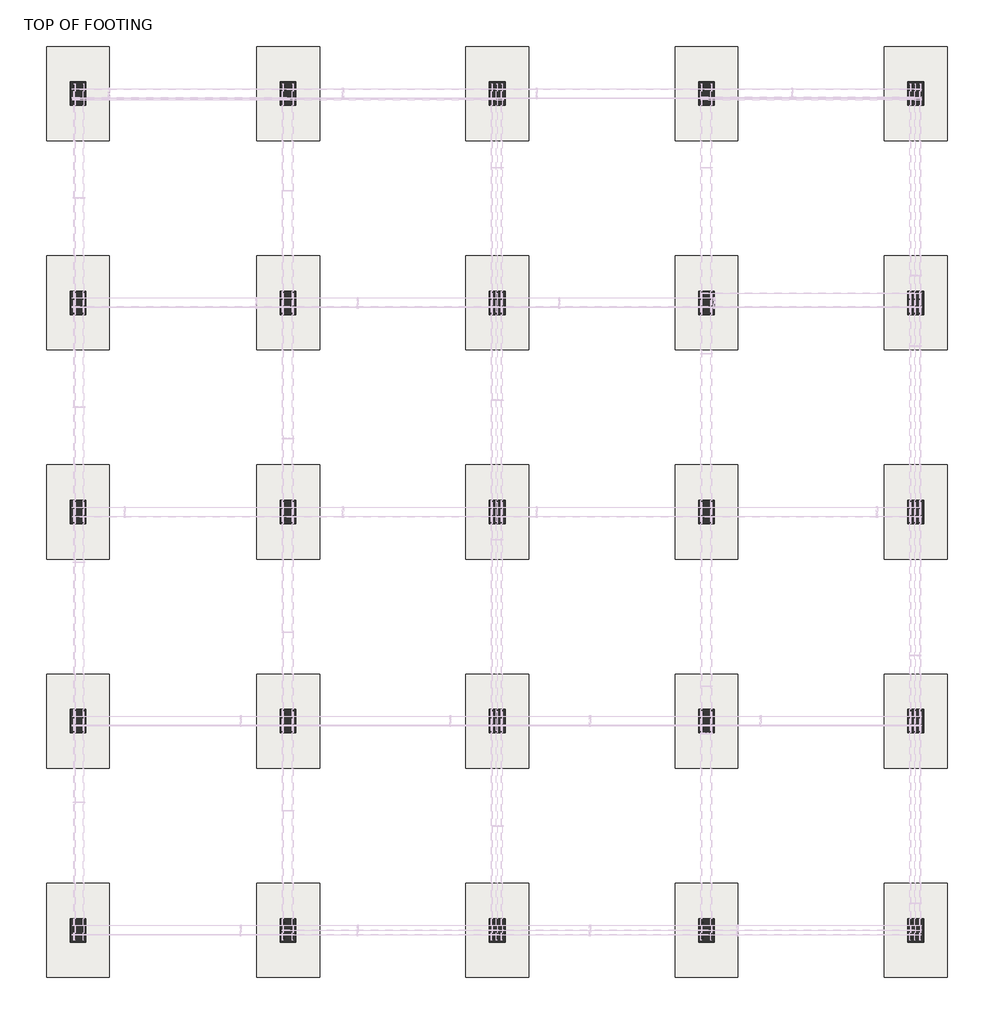
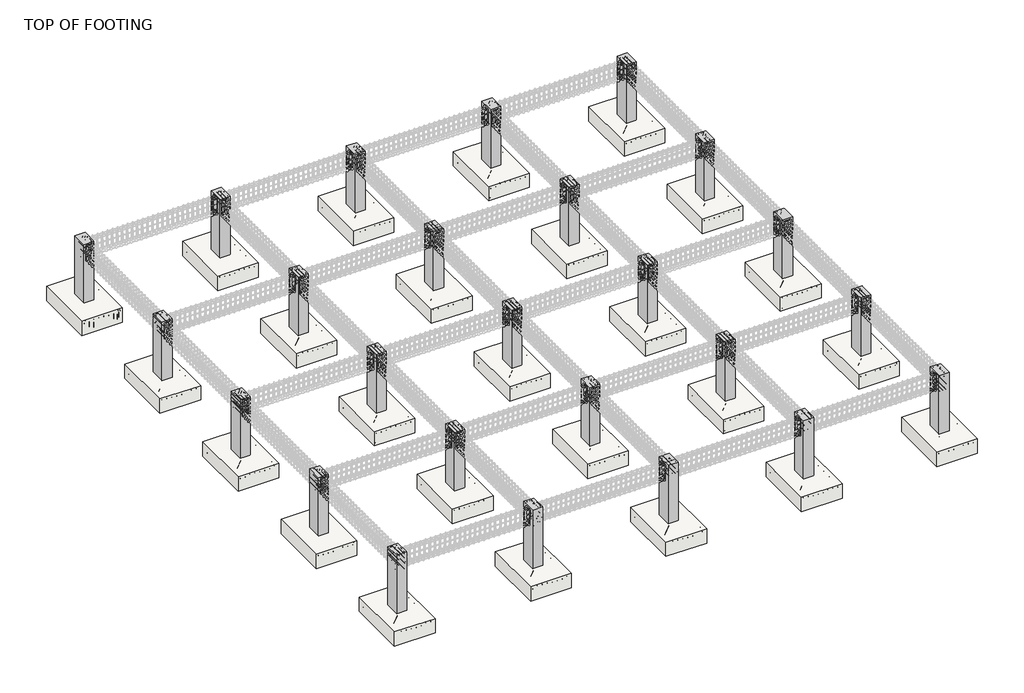
# One storey, part 1 of 21: 25 columns, 25 slabs.
"""IFC4 building model written with IfcOpenShell, lengths in millimetres."""

from ifc_helpers import new_model, si_unit, frame, origin, place, context, project, spatial, polyline, outline, extrude, faceted_brep, transform, mapped, element, save
from components import m_footing_rectangular_1800_x_1200_x_450mm_16ba7ea5

model = new_model("IFC4")

# Units and contexts
model_context = context("Model", 3, world=origin())
ifc_project = project(units=[si_unit("LENGTHUNIT", "METRE", prefix="MILLI")], contexts=[model_context])

# Site, building, storey
site = spatial("IfcSite", under=ifc_project)
building = spatial("IfcBuilding", under=site)
storey = spatial("IfcBuildingStorey", under=building, Name="TOP OF FOOTING", Elevation=-1828.8)

# Columns
placement = place(None, origin())
element("IfcColumn", 1, ObjectType="M_Concrete-Rectangular-Column : 300 x 450mm", at=placement, inside=storey, context=model_context, shape_type="SweptSolid", body=[
    extrude(outline(polyline([(-13671.9084825, 15814.5386958), (-13671.9084825, 15364.5386958), (-13971.9084825, 15364.5386958), (-13971.9084825, 15814.5386958), (-13671.9084825, 15814.5386958)])), frame((0.0, 0.0, -1828.8), z_axis=(0.0, 0.0, 1.0), x_axis=(1.0, 0.0, 0.0)), (0.0, 0.0, 1.0), 1828.8),
])
element("IfcColumn", 2, ObjectType="M_Concrete-Rectangular-Column : 300 x 450mm", at=placement, inside=storey, context=model_context, shape_type="Brep", body=[
    faceted_brep([(-9652.1813539, 15814.5386958, -1828.8), (-9652.1813539, 15364.5386958, -1828.8), (-9952.1813539, 15364.5386958, -1828.8), (-9952.1813539, 15814.5386958, -1828.8), (-9652.1813539, 15814.5386958, 0.0), (-9652.1813539, 15439.5386958, 0.0), (-9652.1813539, 15364.5386958, 0.0), (-9952.1813539, 15364.5386958, 0.0), (-9952.1813539, 15439.5386958, 0.0), (-9952.1813539, 15814.5386958, 0.0)], [[[0, 1, 2, 3]], [[4, 5, 6, 1, 0]], [[6, 7, 2, 1]], [[7, 8, 9, 3, 2]], [[9, 4, 0, 3]], [[4, 9, 8, 7, 6, 5]]]),
])
element("IfcColumn", 3, ObjectType="M_Concrete-Rectangular-Column : 300 x 450mm", at=placement, inside=storey, context=model_context, shape_type="Brep", body=[
    faceted_brep([(-5652.1813539, 15814.5386958, -1828.8), (-5652.1813539, 15364.5386958, -1828.8), (-5952.1813539, 15364.5386958, -1828.8), (-5952.1813539, 15814.5386958, -1828.8), (-5652.1813539, 15814.5386958, 0.0), (-5652.1813539, 15439.5386958, 0.0), (-5652.1813539, 15364.5386958, 0.0), (-5952.1813539, 15364.5386958, 0.0), (-5952.1813539, 15439.5386958, 0.0), (-5952.1813539, 15814.5386958, 0.0)], [[[0, 1, 2, 3]], [[4, 5, 6, 1, 0]], [[6, 7, 2, 1]], [[7, 8, 9, 3, 2]], [[9, 4, 0, 3]], [[4, 9, 8, 7, 6, 5]]]),
])
element("IfcColumn", 4, ObjectType="M_Concrete-Rectangular-Column : 300 x 450mm", at=placement, inside=storey, context=model_context, shape_type="Brep", body=[
    faceted_brep([(-1652.1813539, 15814.5386958, -1828.8), (-1652.1813539, 15364.5386958, -1828.8), (-1952.1813539, 15364.5386958, -1828.8), (-1952.1813539, 15814.5386958, -1828.8), (-1652.1813539, 15814.5386958, 0.0), (-1652.1813539, 15439.5386958, 0.0), (-1652.1813539, 15364.5386958, 0.0), (-1952.1813539, 15364.5386958, 0.0), (-1952.1813539, 15439.5386958, 0.0), (-1952.1813539, 15814.5386958, 0.0)], [[[0, 1, 2, 3]], [[4, 5, 6, 1, 0]], [[6, 7, 2, 1]], [[7, 8, 9, 3, 2]], [[9, 4, 0, 3]], [[4, 9, 8, 7, 6, 5]]]),
])
element("IfcColumn", 5, ObjectType="M_Concrete-Rectangular-Column : 300 x 450mm", at=placement, inside=storey, context=model_context, shape_type="Brep", body=[
    faceted_brep([(2347.8186461, 15814.5386958, -1828.8), (2347.8186461, 15364.5386958, -1828.8), (2047.8186461, 15364.5386958, -1828.8), (2047.8186461, 15814.5386958, -1828.8), (2347.8186461, 15814.5386958, 0.0), (2347.8186461, 15364.5386958, 0.0), (2047.8186461, 15364.5386958, 0.0), (2047.8186461, 15439.5386958, 0.0), (2047.8186461, 15814.5386958, 0.0)], [[[0, 1, 2, 3]], [[4, 5, 1, 0]], [[5, 6, 2, 1]], [[6, 7, 8, 3, 2]], [[8, 4, 0, 3]], [[4, 8, 7, 6, 5]]]),
])
element("IfcColumn", 6, ObjectType="M_Concrete-Rectangular-Column : 300 x 450mm", at=placement, inside=storey, context=model_context, shape_type="SweptSolid", body=[
    extrude(outline(polyline([(-13671.9084825, 11814.5386958), (-13671.9084825, 11364.5386958), (-13971.9084825, 11364.5386958), (-13971.9084825, 11814.5386958), (-13671.9084825, 11814.5386958)])), frame((0.0, 0.0, -1828.8), z_axis=(0.0, 0.0, 1.0), x_axis=(1.0, 0.0, 0.0)), (0.0, 0.0, 1.0), 1828.8),
])
element("IfcColumn", 7, ObjectType="M_Concrete-Rectangular-Column : 300 x 450mm", at=placement, inside=storey, context=model_context, shape_type="Brep", body=[
    faceted_brep([(-9652.1813539, 11814.5386958, -1828.8), (-9652.1813539, 11364.5386958, -1828.8), (-9952.1813539, 11364.5386958, -1828.8), (-9952.1813539, 11814.5386958, -1828.8), (-9652.1813539, 11814.5386958, 0.0), (-9652.1813539, 11739.5386958, 0.0), (-9652.1813539, 11439.5386958, 0.0), (-9652.1813539, 11364.5386958, 0.0), (-9952.1813539, 11364.5386958, 0.0), (-9952.1813539, 11439.5386958, 0.0), (-9952.1813539, 11739.5386958, 0.0), (-9952.1813539, 11814.5386958, 0.0)], [[[0, 1, 2, 3]], [[4, 5, 6, 7, 1, 0]], [[7, 8, 2, 1]], [[8, 9, 10, 11, 3, 2]], [[11, 4, 0, 3]], [[4, 11, 10, 9, 8, 7, 6, 5]]]),
])
element("IfcColumn", 8, ObjectType="M_Concrete-Rectangular-Column : 300 x 450mm", at=placement, inside=storey, context=model_context, shape_type="Brep", body=[
    faceted_brep([(-5652.1813539, 11814.5386958, -1828.8), (-5652.1813539, 11364.5386958, -1828.8), (-5952.1813539, 11364.5386958, -1828.8), (-5952.1813539, 11814.5386958, -1828.8), (-5652.1813539, 11814.5386958, 0.0), (-5652.1813539, 11739.5386958, 0.0), (-5652.1813539, 11439.5386958, 0.0), (-5652.1813539, 11364.5386958, 0.0), (-5952.1813539, 11364.5386958, 0.0), (-5952.1813539, 11439.5386958, 0.0), (-5952.1813539, 11739.5386958, 0.0), (-5952.1813539, 11814.5386958, 0.0)], [[[0, 1, 2, 3]], [[4, 5, 6, 7, 1, 0]], [[7, 8, 2, 1]], [[8, 9, 10, 11, 3, 2]], [[11, 4, 0, 3]], [[4, 11, 10, 9, 8, 7, 6, 5]]]),
])
element("IfcColumn", 9, ObjectType="M_Concrete-Rectangular-Column : 300 x 450mm", at=placement, inside=storey, context=model_context, shape_type="Brep", body=[
    faceted_brep([(-1652.1813539, 11814.5386958, -1828.8), (-1652.1813539, 11364.5386958, -1828.8), (-1952.1813539, 11364.5386958, -1828.8), (-1952.1813539, 11814.5386958, -1828.8), (-1652.1813539, 11814.5386958, 0.0), (-1652.1813539, 11739.5386958, 0.0), (-1652.1813539, 11419.5386958, 0.0), (-1652.1813539, 11364.5386958, 0.0), (-1952.1813539, 11364.5386958, 0.0), (-1952.1813539, 11439.5386958, 0.0), (-1952.1813539, 11739.5386958, 0.0), (-1952.1813539, 11814.5386958, 0.0)], [[[0, 1, 2, 3]], [[4, 5, 6, 7, 1, 0]], [[7, 8, 2, 1]], [[8, 9, 10, 11, 3, 2]], [[11, 4, 0, 3]], [[4, 11, 10, 9, 8, 7, 6, 5]]]),
])
element("IfcColumn", 10, ObjectType="M_Concrete-Rectangular-Column : 300 x 450mm", at=placement, inside=storey, context=model_context, shape_type="Brep", body=[
    faceted_brep([(2347.8186461, 11814.5386958, -1828.8), (2347.8186461, 11364.5386958, -1828.8), (2047.8186461, 11364.5386958, -1828.8), (2047.8186461, 11814.5386958, -1828.8), (2347.8186461, 11814.5386958, 0.0), (2347.8186461, 11774.5386958, 0.0), (2347.8186461, 11364.5386958, 0.0), (2047.8186461, 11364.5386958, 0.0), (2047.8186461, 11419.5386958, 0.0), (2047.8186461, 11739.5386958, 0.0), (2047.8186461, 11814.5386958, 0.0)], [[[0, 1, 2, 3]], [[4, 5, 6, 1, 0]], [[6, 7, 2, 1]], [[7, 8, 9, 10, 3, 2]], [[10, 4, 0, 3]], [[4, 10, 9, 8, 7, 6, 5]]]),
])
element("IfcColumn", 11, ObjectType="M_Concrete-Rectangular-Column : 300 x 450mm", at=placement, inside=storey, context=model_context, shape_type="SweptSolid", body=[
    extrude(outline(polyline([(-13671.9084825, 7814.5386958), (-13671.9084825, 7364.5386958), (-13971.9084825, 7364.5386958), (-13971.9084825, 7814.5386958), (-13671.9084825, 7814.5386958)])), frame((0.0, 0.0, -1828.8), z_axis=(0.0, 0.0, 1.0), x_axis=(1.0, 0.0, 0.0)), (0.0, 0.0, 1.0), 1828.8),
])
element("IfcColumn", 12, ObjectType="M_Concrete-Rectangular-Column : 300 x 450mm", at=placement, inside=storey, context=model_context, shape_type="Brep", body=[
    faceted_brep([(-9652.1813539, 7814.5386958, -1828.8), (-9652.1813539, 7364.5386958, -1828.8), (-9952.1813539, 7364.5386958, -1828.8), (-9952.1813539, 7814.5386958, -1828.8), (-9652.1813539, 7814.5386958, 0.0), (-9652.1813539, 7739.5386958, 0.0), (-9652.1813539, 7439.5386958, 0.0), (-9652.1813539, 7364.5386958, 0.0), (-9952.1813539, 7364.5386958, 0.0), (-9952.1813539, 7439.5386958, 0.0), (-9952.1813539, 7739.5386958, 0.0), (-9952.1813539, 7814.5386958, 0.0)], [[[0, 1, 2, 3]], [[4, 5, 6, 7, 1, 0]], [[7, 8, 2, 1]], [[8, 9, 10, 11, 3, 2]], [[11, 4, 0, 3]], [[4, 11, 10, 9, 8, 7, 6, 5]]]),
])
element("IfcColumn", 13, ObjectType="M_Concrete-Rectangular-Column : 300 x 450mm", at=placement, inside=storey, context=model_context, shape_type="Brep", body=[
    faceted_brep([(-5652.1813539, 7814.5386958, -1828.8), (-5652.1813539, 7364.5386958, -1828.8), (-5952.1813539, 7364.5386958, -1828.8), (-5952.1813539, 7814.5386958, -1828.8), (-5652.1813539, 7814.5386958, 0.0), (-5652.1813539, 7739.5386958, 0.0), (-5652.1813539, 7439.5386958, 0.0), (-5652.1813539, 7364.5386958, 0.0), (-5952.1813539, 7364.5386958, 0.0), (-5952.1813539, 7439.5386958, 0.0), (-5952.1813539, 7739.5386958, 0.0), (-5952.1813539, 7814.5386958, 0.0)], [[[0, 1, 2, 3]], [[4, 5, 6, 7, 1, 0]], [[7, 8, 2, 1]], [[8, 9, 10, 11, 3, 2]], [[11, 4, 0, 3]], [[4, 11, 10, 9, 8, 7, 6, 5]]]),
])
element("IfcColumn", 14, ObjectType="M_Concrete-Rectangular-Column : 300 x 450mm", at=placement, inside=storey, context=model_context, shape_type="Brep", body=[
    faceted_brep([(-1652.1813539, 7814.5386958, -1828.8), (-1652.1813539, 7364.5386958, -1828.8), (-1952.1813539, 7364.5386958, -1828.8), (-1952.1813539, 7814.5386958, -1828.8), (-1652.1813539, 7814.5386958, 0.0), (-1652.1813539, 7719.5386958, 0.0), (-1652.1813539, 7439.5386958, 0.0), (-1652.1813539, 7364.5386958, 0.0), (-1952.1813539, 7364.5386958, 0.0), (-1952.1813539, 7439.5386958, 0.0), (-1952.1813539, 7739.5386958, 0.0), (-1952.1813539, 7814.5386958, 0.0)], [[[0, 1, 2, 3]], [[4, 5, 6, 7, 1, 0]], [[7, 8, 2, 1]], [[8, 9, 10, 11, 3, 2]], [[11, 4, 0, 3]], [[4, 11, 10, 9, 8, 7, 6, 5]]]),
])
element("IfcColumn", 15, ObjectType="M_Concrete-Rectangular-Column : 300 x 450mm", at=placement, inside=storey, context=model_context, shape_type="Brep", body=[
    faceted_brep([(2347.8186461, 7814.5386958, -1828.8), (2347.8186461, 7364.5386958, -1828.8), (2047.8186461, 7364.5386958, -1828.8), (2047.8186461, 7814.5386958, -1828.8), (2347.8186461, 7814.5386958, 0.0), (2347.8186461, 7774.5386958, 0.0), (2347.8186461, 7364.5386958, 0.0), (2047.8186461, 7364.5386958, 0.0), (2047.8186461, 7439.5386958, 0.0), (2047.8186461, 7719.5386958, 0.0), (2047.8186461, 7814.5386958, 0.0)], [[[0, 1, 2, 3]], [[4, 5, 6, 1, 0]], [[6, 7, 2, 1]], [[7, 8, 9, 10, 3, 2]], [[10, 4, 0, 3]], [[4, 10, 9, 8, 7, 6, 5]]]),
])
element("IfcColumn", 16, ObjectType="M_Concrete-Rectangular-Column : 300 x 450mm", at=placement, inside=storey, context=model_context, shape_type="SweptSolid", body=[
    extrude(outline(polyline([(-13671.9084825, 3814.5386958), (-13671.9084825, 3364.5386958), (-13971.9084825, 3364.5386958), (-13971.9084825, 3814.5386958), (-13671.9084825, 3814.5386958)])), frame((0.0, 0.0, -1828.8), z_axis=(0.0, 0.0, 1.0), x_axis=(1.0, 0.0, 0.0)), (0.0, 0.0, 1.0), 1828.8),
])
element("IfcColumn", 17, ObjectType="M_Concrete-Rectangular-Column : 300 x 450mm", at=placement, inside=storey, context=model_context, shape_type="Brep", body=[
    faceted_brep([(-9652.1813539, 3814.5386958, -1828.8), (-9652.1813539, 3364.5386958, -1828.8), (-9952.1813539, 3364.5386958, -1828.8), (-9952.1813539, 3814.5386958, -1828.8), (-9652.1813539, 3814.5386958, 0.0), (-9652.1813539, 3739.5386958, 0.0), (-9652.1813539, 3439.5386958, 0.0), (-9652.1813539, 3364.5386958, 0.0), (-9952.1813539, 3364.5386958, 0.0), (-9952.1813539, 3439.5386958, 0.0), (-9952.1813539, 3739.5386958, 0.0), (-9952.1813539, 3814.5386958, 0.0)], [[[0, 1, 2, 3]], [[4, 5, 6, 7, 1, 0]], [[7, 8, 2, 1]], [[8, 9, 10, 11, 3, 2]], [[11, 4, 0, 3]], [[4, 11, 10, 9, 8, 7, 6, 5]]]),
])
element("IfcColumn", 18, ObjectType="M_Concrete-Rectangular-Column : 300 x 450mm", at=placement, inside=storey, context=model_context, shape_type="Brep", body=[
    faceted_brep([(-5652.1813539, 3814.5386958, -1828.8), (-5652.1813539, 3364.5386958, -1828.8), (-5952.1813539, 3364.5386958, -1828.8), (-5952.1813539, 3814.5386958, -1828.8), (-5652.1813539, 3814.5386958, 0.0), (-5652.1813539, 3739.5386958, 0.0), (-5652.1813539, 3439.5386958, 0.0), (-5652.1813539, 3364.5386958, 0.0), (-5952.1813539, 3364.5386958, 0.0), (-5952.1813539, 3439.5386958, 0.0), (-5952.1813539, 3739.5386958, 0.0), (-5952.1813539, 3814.5386958, 0.0)], [[[0, 1, 2, 3]], [[4, 5, 6, 7, 1, 0]], [[7, 8, 2, 1]], [[8, 9, 10, 11, 3, 2]], [[11, 4, 0, 3]], [[4, 11, 10, 9, 8, 7, 6, 5]]]),
])
element("IfcColumn", 19, ObjectType="M_Concrete-Rectangular-Column : 300 x 450mm", at=placement, inside=storey, context=model_context, shape_type="Brep", body=[
    faceted_brep([(-1652.1813539, 3814.5386958, -1828.8), (-1652.1813539, 3364.5386958, -1828.8), (-1952.1813539, 3364.5386958, -1828.8), (-1952.1813539, 3814.5386958, -1828.8), (-1652.1813539, 3814.5386958, 0.0), (-1652.1813539, 3739.5386958, 0.0), (-1652.1813539, 3439.5386958, 0.0), (-1652.1813539, 3364.5386958, 0.0), (-1952.1813539, 3364.5386958, 0.0), (-1952.1813539, 3439.5386958, 0.0), (-1952.1813539, 3739.5386958, 0.0), (-1952.1813539, 3814.5386958, 0.0)], [[[0, 1, 2, 3]], [[4, 5, 6, 7, 1, 0]], [[7, 8, 2, 1]], [[8, 9, 10, 11, 3, 2]], [[11, 4, 0, 3]], [[4, 11, 10, 9, 8, 7, 6, 5]]]),
])
element("IfcColumn", 20, ObjectType="M_Concrete-Rectangular-Column : 300 x 450mm", at=placement, inside=storey, context=model_context, shape_type="Brep", body=[
    faceted_brep([(2347.8186461, 3814.5386958, -1828.8), (2347.8186461, 3364.5386958, -1828.8), (2047.8186461, 3364.5386958, -1828.8), (2047.8186461, 3814.5386958, -1828.8), (2347.8186461, 3814.5386958, 0.0), (2347.8186461, 3774.5386958, 0.0), (2347.8186461, 3364.5386958, 0.0), (2047.8186461, 3364.5386958, 0.0), (2047.8186461, 3439.5386958, 0.0), (2047.8186461, 3739.5386958, 0.0), (2047.8186461, 3814.5386958, 0.0)], [[[0, 1, 2, 3]], [[4, 5, 6, 1, 0]], [[6, 7, 2, 1]], [[7, 8, 9, 10, 3, 2]], [[10, 4, 0, 3]], [[4, 10, 9, 8, 7, 6, 5]]]),
])
element("IfcColumn", 21, ObjectType="M_Concrete-Rectangular-Column : 300 x 450mm", at=placement, inside=storey, context=model_context, shape_type="SweptSolid", body=[
    extrude(outline(polyline([(-13671.9084825, -185.4613042), (-13671.9084825, -635.4613042), (-13971.9084825, -635.4613042), (-13971.9084825, -185.4613042), (-13671.9084825, -185.4613042)])), frame((0.0, 0.0, -1828.8), z_axis=(0.0, 0.0, 1.0), x_axis=(1.0, 0.0, 0.0)), (0.0, 0.0, 1.0), 1828.8),
])
element("IfcColumn", 22, ObjectType="M_Concrete-Rectangular-Column : 300 x 450mm", at=placement, inside=storey, context=model_context, shape_type="Brep", body=[
    faceted_brep([(-9652.1813539, -185.4613042, -1828.8), (-9652.1813539, -635.4613042, -1828.8), (-9952.1813539, -635.4613042, -1828.8), (-9952.1813539, -185.4613042, -1828.8), (-9652.1813539, -185.4613042, 0.0), (-9652.1813539, -260.4613042, 0.0), (-9652.1813539, -635.4613042, 0.0), (-9952.1813539, -635.4613042, 0.0), (-9952.1813539, -260.4613042, 0.0), (-9952.1813539, -185.4613042, 0.0)], [[[0, 1, 2, 3]], [[4, 5, 6, 1, 0]], [[6, 7, 2, 1]], [[7, 8, 9, 3, 2]], [[9, 4, 0, 3]], [[4, 9, 8, 7, 6, 5]]]),
])
element("IfcColumn", 23, ObjectType="M_Concrete-Rectangular-Column : 300 x 450mm", at=placement, inside=storey, context=model_context, shape_type="Brep", body=[
    faceted_brep([(-5652.1813539, -185.4613042, -1828.8), (-5652.1813539, -635.4613042, -1828.8), (-5952.1813539, -635.4613042, -1828.8), (-5952.1813539, -185.4613042, -1828.8), (-5652.1813539, -185.4613042, 0.0), (-5652.1813539, -260.4613042, 0.0), (-5652.1813539, -635.4613042, 0.0), (-5952.1813539, -635.4613042, 0.0), (-5952.1813539, -260.4613042, 0.0), (-5952.1813539, -185.4613042, 0.0)], [[[0, 1, 2, 3]], [[4, 5, 6, 1, 0]], [[6, 7, 2, 1]], [[7, 8, 9, 3, 2]], [[9, 4, 0, 3]], [[4, 9, 8, 7, 6, 5]]]),
])
element("IfcColumn", 24, ObjectType="M_Concrete-Rectangular-Column : 300 x 450mm", at=placement, inside=storey, context=model_context, shape_type="Brep", body=[
    faceted_brep([(-1652.1813539, -185.4613042, -1828.8), (-1652.1813539, -635.4613042, -1828.8), (-1952.1813539, -635.4613042, -1828.8), (-1952.1813539, -185.4613042, -1828.8), (-1652.1813539, -185.4613042, 0.0), (-1652.1813539, -260.4613042, 0.0), (-1652.1813539, -635.4613042, 0.0), (-1952.1813539, -635.4613042, 0.0), (-1952.1813539, -260.4613042, 0.0), (-1952.1813539, -185.4613042, 0.0)], [[[0, 1, 2, 3]], [[4, 5, 6, 1, 0]], [[6, 7, 2, 1]], [[7, 8, 9, 3, 2]], [[9, 4, 0, 3]], [[4, 9, 8, 7, 6, 5]]]),
])
element("IfcColumn", 25, ObjectType="M_Concrete-Rectangular-Column : 300 x 450mm", at=placement, inside=storey, context=model_context, shape_type="Brep", body=[
    faceted_brep([(2347.8186461, -185.4613042, -1828.8), (2347.8186461, -635.4613042, -1828.8), (2047.8186461, -635.4613042, -1828.8), (2047.8186461, -185.4613042, -1828.8), (2347.8186461, -185.4613042, 0.0), (2347.8186461, -225.4613042, 0.0), (2347.8186461, -635.4613042, 0.0), (2047.8186461, -635.4613042, 0.0), (2047.8186461, -260.4613042, 0.0), (2047.8186461, -185.4613042, 0.0)], [[[0, 1, 2, 3]], [[4, 5, 6, 1, 0]], [[6, 7, 2, 1]], [[7, 8, 9, 3, 2]], [[9, 4, 0, 3]], [[4, 9, 8, 7, 6, 5]]]),
])

# Slabs
m_footing_rectangular_1800_x_1200_x_450mm_shape = m_footing_rectangular_1800_x_1200_x_450mm_16ba7ea5(model_context)
element("IfcSlab", 26, ObjectType="M_Footing-Rectangular : 1800 x 1200 x 450mm", at=placement, inside=storey, context=model_context, shape_type="MappedRepresentation", body=[
    mapped(m_footing_rectangular_1800_x_1200_x_450mm_shape, transform((-13821.9084825, 15589.5386958, -1828.8), x_axis=(1.0, 0.0, 0.0), y_axis=(0.0, 1.0, 0.0), z_axis=(0.0, 0.0, 1.0))),
])
element("IfcSlab", 27, ObjectType="M_Footing-Rectangular : 1800 x 1200 x 450mm", at=placement, inside=storey, context=model_context, shape_type="MappedRepresentation", body=[
    mapped(m_footing_rectangular_1800_x_1200_x_450mm_shape, transform((-9802.1813539, 15589.5386958, -1828.8), x_axis=(1.0, 0.0, 0.0), y_axis=(0.0, 1.0, 0.0), z_axis=(0.0, 0.0, 1.0))),
])
element("IfcSlab", 28, ObjectType="M_Footing-Rectangular : 1800 x 1200 x 450mm", at=placement, inside=storey, context=model_context, shape_type="MappedRepresentation", body=[
    mapped(m_footing_rectangular_1800_x_1200_x_450mm_shape, transform((-5802.1813539, 15589.5386958, -1828.8), x_axis=(1.0, 0.0, 0.0), y_axis=(0.0, 1.0, 0.0), z_axis=(0.0, 0.0, 1.0))),
])
element("IfcSlab", 29, ObjectType="M_Footing-Rectangular : 1800 x 1200 x 450mm", at=placement, inside=storey, context=model_context, shape_type="MappedRepresentation", body=[
    mapped(m_footing_rectangular_1800_x_1200_x_450mm_shape, transform((-1802.1813539, 15589.5386958, -1828.8), x_axis=(1.0, 0.0, 0.0), y_axis=(0.0, 1.0, 0.0), z_axis=(0.0, 0.0, 1.0))),
])
element("IfcSlab", 30, ObjectType="M_Footing-Rectangular : 1800 x 1200 x 450mm", at=placement, inside=storey, context=model_context, shape_type="MappedRepresentation", body=[
    mapped(m_footing_rectangular_1800_x_1200_x_450mm_shape, transform((2197.8186461, 15589.5386958, -1828.8), x_axis=(1.0, 0.0, 0.0), y_axis=(0.0, 1.0, 0.0), z_axis=(0.0, 0.0, 1.0))),
])
element("IfcSlab", 31, ObjectType="M_Footing-Rectangular : 1800 x 1200 x 450mm", at=placement, inside=storey, context=model_context, shape_type="MappedRepresentation", body=[
    mapped(m_footing_rectangular_1800_x_1200_x_450mm_shape, transform((2197.8186461, 11589.5386958, -1828.8), x_axis=(1.0, 0.0, 0.0), y_axis=(0.0, 1.0, 0.0), z_axis=(0.0, 0.0, 1.0))),
])
element("IfcSlab", 32, ObjectType="M_Footing-Rectangular : 1800 x 1200 x 450mm", at=placement, inside=storey, context=model_context, shape_type="MappedRepresentation", body=[
    mapped(m_footing_rectangular_1800_x_1200_x_450mm_shape, transform((-1802.1813539, 11589.5386958, -1828.8), x_axis=(1.0, 0.0, 0.0), y_axis=(0.0, 1.0, 0.0), z_axis=(0.0, 0.0, 1.0))),
])
element("IfcSlab", 33, ObjectType="M_Footing-Rectangular : 1800 x 1200 x 450mm", at=placement, inside=storey, context=model_context, shape_type="MappedRepresentation", body=[
    mapped(m_footing_rectangular_1800_x_1200_x_450mm_shape, transform((-5802.1813539, 11589.5386958, -1828.8), x_axis=(1.0, 0.0, 0.0), y_axis=(0.0, 1.0, 0.0), z_axis=(0.0, 0.0, 1.0))),
])
element("IfcSlab", 34, ObjectType="M_Footing-Rectangular : 1800 x 1200 x 450mm", at=placement, inside=storey, context=model_context, shape_type="MappedRepresentation", body=[
    mapped(m_footing_rectangular_1800_x_1200_x_450mm_shape, transform((-9802.1813539, 11589.5386958, -1828.8), x_axis=(1.0, 0.0, 0.0), y_axis=(0.0, 1.0, 0.0), z_axis=(0.0, 0.0, 1.0))),
])
element("IfcSlab", 35, ObjectType="M_Footing-Rectangular : 1800 x 1200 x 450mm", at=placement, inside=storey, context=model_context, shape_type="MappedRepresentation", body=[
    mapped(m_footing_rectangular_1800_x_1200_x_450mm_shape, transform((-13821.9084825, 11589.5386958, -1828.8), x_axis=(1.0, 0.0, 0.0), y_axis=(0.0, 1.0, 0.0), z_axis=(0.0, 0.0, 1.0))),
])
element("IfcSlab", 36, ObjectType="M_Footing-Rectangular : 1800 x 1200 x 450mm", at=placement, inside=storey, context=model_context, shape_type="MappedRepresentation", body=[
    mapped(m_footing_rectangular_1800_x_1200_x_450mm_shape, transform((-13821.9084825, -410.4613042, -1828.8), x_axis=(1.0, 0.0, 0.0), y_axis=(0.0, 1.0, 0.0), z_axis=(0.0, 0.0, 1.0))),
])
element("IfcSlab", 37, ObjectType="M_Footing-Rectangular : 1800 x 1200 x 450mm", at=placement, inside=storey, context=model_context, shape_type="MappedRepresentation", body=[
    mapped(m_footing_rectangular_1800_x_1200_x_450mm_shape, transform((-9802.1813539, -410.4613042, -1828.8), x_axis=(1.0, 0.0, 0.0), y_axis=(0.0, 1.0, 0.0), z_axis=(0.0, 0.0, 1.0))),
])
element("IfcSlab", 38, ObjectType="M_Footing-Rectangular : 1800 x 1200 x 450mm", at=placement, inside=storey, context=model_context, shape_type="MappedRepresentation", body=[
    mapped(m_footing_rectangular_1800_x_1200_x_450mm_shape, transform((-5802.1813539, -410.4613042, -1828.8), x_axis=(1.0, 0.0, 0.0), y_axis=(0.0, 1.0, 0.0), z_axis=(0.0, 0.0, 1.0))),
])
element("IfcSlab", 39, ObjectType="M_Footing-Rectangular : 1800 x 1200 x 450mm", at=placement, inside=storey, context=model_context, shape_type="MappedRepresentation", body=[
    mapped(m_footing_rectangular_1800_x_1200_x_450mm_shape, transform((-1802.1813539, -410.4613042, -1828.8), x_axis=(1.0, 0.0, 0.0), y_axis=(0.0, 1.0, 0.0), z_axis=(0.0, 0.0, 1.0))),
])
element("IfcSlab", 40, ObjectType="M_Footing-Rectangular : 1800 x 1200 x 450mm", at=placement, inside=storey, context=model_context, shape_type="MappedRepresentation", body=[
    mapped(m_footing_rectangular_1800_x_1200_x_450mm_shape, transform((2197.8186461, -410.4613042, -1828.8), x_axis=(1.0, 0.0, 0.0), y_axis=(0.0, 1.0, 0.0), z_axis=(0.0, 0.0, 1.0))),
])
element("IfcSlab", 41, ObjectType="M_Footing-Rectangular : 1800 x 1200 x 450mm", at=placement, inside=storey, context=model_context, shape_type="MappedRepresentation", body=[
    mapped(m_footing_rectangular_1800_x_1200_x_450mm_shape, transform((2197.8186461, 3589.5386958, -1828.8), x_axis=(1.0, 0.0, 0.0), y_axis=(0.0, 1.0, 0.0), z_axis=(0.0, 0.0, 1.0))),
])
element("IfcSlab", 42, ObjectType="M_Footing-Rectangular : 1800 x 1200 x 450mm", at=placement, inside=storey, context=model_context, shape_type="MappedRepresentation", body=[
    mapped(m_footing_rectangular_1800_x_1200_x_450mm_shape, transform((-1802.1813539, 3589.5386958, -1828.8), x_axis=(1.0, 0.0, 0.0), y_axis=(0.0, 1.0, 0.0), z_axis=(0.0, 0.0, 1.0))),
])
element("IfcSlab", 43, ObjectType="M_Footing-Rectangular : 1800 x 1200 x 450mm", at=placement, inside=storey, context=model_context, shape_type="MappedRepresentation", body=[
    mapped(m_footing_rectangular_1800_x_1200_x_450mm_shape, transform((-5802.1813539, 3589.5386958, -1828.8), x_axis=(1.0, 0.0, 0.0), y_axis=(0.0, 1.0, 0.0), z_axis=(0.0, 0.0, 1.0))),
])
element("IfcSlab", 44, ObjectType="M_Footing-Rectangular : 1800 x 1200 x 450mm", at=placement, inside=storey, context=model_context, shape_type="MappedRepresentation", body=[
    mapped(m_footing_rectangular_1800_x_1200_x_450mm_shape, transform((-9802.1813539, 3589.5386958, -1828.8), x_axis=(1.0, 0.0, 0.0), y_axis=(0.0, 1.0, 0.0), z_axis=(0.0, 0.0, 1.0))),
])
element("IfcSlab", 45, ObjectType="M_Footing-Rectangular : 1800 x 1200 x 450mm", at=placement, inside=storey, context=model_context, shape_type="MappedRepresentation", body=[
    mapped(m_footing_rectangular_1800_x_1200_x_450mm_shape, transform((-13821.9084825, 3589.5386958, -1828.8), x_axis=(1.0, 0.0, 0.0), y_axis=(0.0, 1.0, 0.0), z_axis=(0.0, 0.0, 1.0))),
])
element("IfcSlab", 46, ObjectType="M_Footing-Rectangular : 1800 x 1200 x 450mm", at=placement, inside=storey, context=model_context, shape_type="MappedRepresentation", body=[
    mapped(m_footing_rectangular_1800_x_1200_x_450mm_shape, transform((-13821.9084825, 7589.5386958, -1828.8), x_axis=(1.0, 0.0, 0.0), y_axis=(0.0, 1.0, 0.0), z_axis=(0.0, 0.0, 1.0))),
])
element("IfcSlab", 47, ObjectType="M_Footing-Rectangular : 1800 x 1200 x 450mm", at=placement, inside=storey, context=model_context, shape_type="MappedRepresentation", body=[
    mapped(m_footing_rectangular_1800_x_1200_x_450mm_shape, transform((-9802.1813539, 7589.5386958, -1828.8), x_axis=(1.0, 0.0, 0.0), y_axis=(0.0, 1.0, 0.0), z_axis=(0.0, 0.0, 1.0))),
])
element("IfcSlab", 48, ObjectType="M_Footing-Rectangular : 1800 x 1200 x 450mm", at=placement, inside=storey, context=model_context, shape_type="MappedRepresentation", body=[
    mapped(m_footing_rectangular_1800_x_1200_x_450mm_shape, transform((-5802.1813539, 7589.5386958, -1828.8), x_axis=(1.0, 0.0, 0.0), y_axis=(0.0, 1.0, 0.0), z_axis=(0.0, 0.0, 1.0))),
])
element("IfcSlab", 49, ObjectType="M_Footing-Rectangular : 1800 x 1200 x 450mm", at=placement, inside=storey, context=model_context, shape_type="MappedRepresentation", body=[
    mapped(m_footing_rectangular_1800_x_1200_x_450mm_shape, transform((-1802.1813539, 7589.5386958, -1828.8), x_axis=(1.0, 0.0, 0.0), y_axis=(0.0, 1.0, 0.0), z_axis=(0.0, 0.0, 1.0))),
])
element("IfcSlab", 50, ObjectType="M_Footing-Rectangular : 1800 x 1200 x 450mm", at=placement, inside=storey, context=model_context, shape_type="MappedRepresentation", body=[
    mapped(m_footing_rectangular_1800_x_1200_x_450mm_shape, transform((2197.8186461, 7589.5386958, -1828.8), x_axis=(1.0, 0.0, 0.0), y_axis=(0.0, 1.0, 0.0), z_axis=(0.0, 0.0, 1.0))),
])

save(model, "model.ifc")

# Revit data of these elements
# Grids (mm)
#   "1": line (-13821.908, 19424.096) -> (-13821.908, -11809.361)
#   "2": line (-9802.181, 19424.096) -> (-9802.181, -11809.361)
#   "3": line (-5802.181, 19424.096) -> (-5802.181, -11809.361)
#   "4": line (-1802.181, 19424.096) -> (-1802.181, -11809.361)
#   "5": line (2197.819, 19424.096) -> (2197.819, -11809.361)
#   "A": line (5218.971, 15589.539) -> (-16500.882, 15589.539)
#   "B": line (5218.971, 11589.539) -> (-16500.882, 11589.539)
#   "C": line (5218.971, 7589.539) -> (-16500.882, 7589.539)
#   "D": line (5218.971, 3589.539) -> (-16500.882, 3589.539)
#   "E": line (5218.971, -410.461) -> (-16500.882, -410.461)
# Type "M_Concrete-Rectangular-Column : 300 x 450mm"
#   b = 0' - 11.81102"
#   h = 1' - 5.71654"
#   Structural Material [instance default] = Concrete, Cast-in-Place gray
# Type "M_Footing-Rectangular : 1800 x 1200 x 450mm"
#   Width = 3' - 11.24409"
#   Length = 5' - 10.86614"
#   Foundation Thickness = 1' - 5.71654"
#   Structural Material [instance default] = Concrete, Cast-in-Place gray
#   Assembly Code = ""
# Elements 1, 2, 3, 4, 5, 6, 7, 8, 9, 10, 11, 12, 13, 14, 15, 16, 17, 18, 19, 20, 21, 22, 23, 24, 25 (IfcColumn, "M_Concrete-Rectangular-Column : 300 x 450mm")
#   Structural Material = Concrete, Cast-in-Place gray
#   Phase Created = New Construction
#   Materials on its faces: "Concrete, Cast-in-Place gray"
# Elements 26, 27, 28, 29, 30, 31, 32, 33, 34, 35, 36, 37, 38, 39, 40, 41, 42, 43, 44, 45, 46, 47, 48, 49, 50 (IfcSlab, "M_Footing-Rectangular : 1800 x 1200 x 450mm")
#   Structural Material = Concrete, Cast-in-Place gray
#   Phase Created = New Construction
#   Materials on its faces: "Concrete, Cast-in-Place gray"
# Materials
#   "Concrete, Cast-in-Place gray": class "Concrete", colour RGB 192 192 192, transparency 0, Description = "Cast-in-place concrete", Cost = 0
